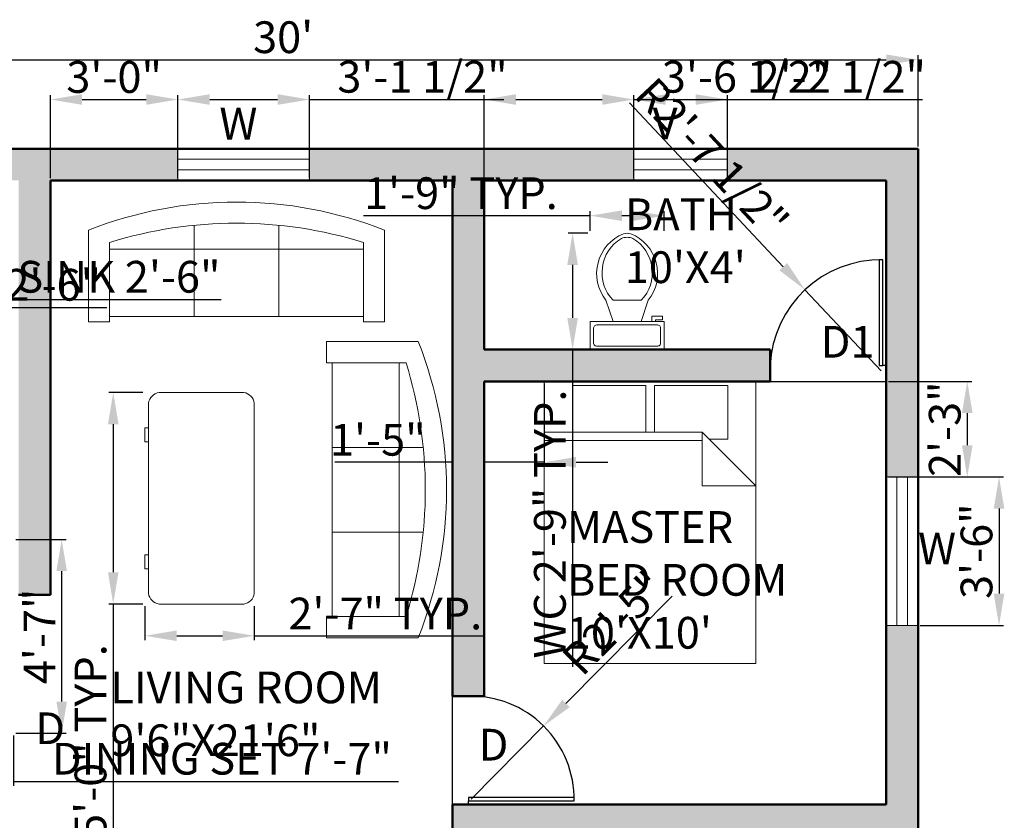
# Model space of a CAD drawing. Units: inches. Extents: x 16989 to 17950, y 7982 to 8536.
# Tile 3 of 5: x 17136 to 17415, y 8270 to 8497. Entities that reach past the tile are written whole.
import ezdxf

# ---------------------------------------------------------------- set-up
doc = ezdxf.new("R2010")
doc.units = ezdxf.units.IN
for name, color, linetype, lineweight in [('A-ANNO-DIMS', 2, 'Continuous', 18), ('A-ANNO-IDEN', 7, 'Continuous', 18), ('A-AREA-IDEN', 7, 'Continuous', 25), ('A-DOOR', 3, 'Continuous', 25), ('A-FLOR-FIXT', 9, 'Continuous', 18), ('A-FURN', 8, 'Continuous', 18), ('A-GLAZ', 4, 'Continuous', 18), ('A-WALL', 7, 'Continuous', 50)]:
    doc.layers.add(name, color=color, linetype=linetype, lineweight=lineweight)
doc.layers.add('A-WALL-PATT', color=177, linetype='Continuous', lineweight=13, true_color=0x293189)
doc.styles.get("Standard").update_dxf_attribs({"font": 'arial.ttf'})
doc.dimstyles.new('ISO-25', dxfattribs={"dimtxt": 9, "dimasz": 9, "dimexe": 1.25, "dimexo": 0.625, "dimtad": 1, "dimdec": 1, "dimrnd": 9, "dimlunit": 3, "dimtxsty": 'Standard', "dimcen": 2.5, "dimadec": 0, "dimazin": 0, "dimtfac": 1, "dimtdec": 1, "dimtmove": 0, "dimatfit": 3, "dimfxl": 1, "dimarcsym": 0})

# ---------------------------------------------------------------- blocks, each defined once
blk = doc.blocks.new('Sofa - Roundback 7 ft.')
for p, q in [((-12.00002, -32.4421), (-12.00003, -6.5971)), ((11.99997, -32.4421), (11.99998, -6.5971)), ((-36.000027, -34), (-36.000027, -11.4696)), ((-35.999844, -13.3819), (35.9998, -13.3819)), ((35.99998, -34), (35.99998, -11.4696)), ((-36.000027, -32.4421), (35.99998, -32.4421))]:
    blk.add_line(p, q)
for points in [[(-36.000027, -34), (-42.000027, -34), (-42.000027, -8)], [(41.99998, -8), (41.99998, -34), (35.99998, -34)]]:
    blk.add_lwpolyline(points)
for centre, radius, start, end in [((0, -114.25), 114.25, 68.43141, 111.5686), ((-0.00001, -127.1968), 121.1968, 72.72033, 107.2797)]:
    blk.add_arc(centre, radius, start, end)
blk = doc.blocks.new('Desk - 30 x 60 in.')
for p, q in [((-26.999995, 0), (26.999995, 0)), ((-29.999995, -27), (-29.999995, -3)), ((29.999995, -3), (29.999995, -27)), ((26.999995, -30), (-26.999995, -30)), ((-20.000005, -30), (-20.000005, -31)), ((-16.000005, -31), (-16.000005, -30)), ((15.999995, -31), (15.999995, -30)), ((19.999995, -30), (19.999995, -31)), ((-20.000005, -31), (-16.000005, -31)), ((19.999995, -31), (15.999995, -31))]:
    blk.add_line(p, q)
for centre, start, end in [((-26.499995, -3.5), 98.1301, 171.8699), ((26.499995, -3.5), 8.130102, 81.8699), ((-26.499995, -26.5), 188.1301, 261.8699), ((26.499995, -26.5), 278.1301, 351.8699)]:
    blk.add_arc(centre, 3.535534, start, end)
blk = doc.blocks.new('Bed - Queen')
for p, q in [((0, -80.00003), (0, 0)), ((0, 0), (59.99999, 0)), ((59.99999, 0), (59.99999, -80.00003)), ((7.99999, -1.2), (28.79998, -1.2)), ((7.99999, -14.4), (7.99999, -1.2)), ((28.79998, -1.2), (28.79998, -14.4)), ((31.19999, -1.2), (51.99999, -1.2)), ((31.19999, -14.4), (31.19999, -1.2)), ((51.99999, -1.2), (51.99999, -16.4)), ((0, -14.4), (44.8, -14.4)), ((59.99999, -29.6), (44.8, -14.4)), ((44.8, -14.4), (44.8, -29.6)), ((51.99999, -16.4), (46.79936, -16.4)), ((44.8, -16.8), (0, -16.8)), ((44.8, -29.6), (59.99999, -29.6)), ((59.99999, -80.00003), (0, -80.00003))]:
    blk.add_line(p, q)
blk = doc.blocks.new('Toilet - top')
for p, q in [((9.5, -6), (9.5, -2)), ((-8, -8.5), (-8, -8)), ((-7, -8), (-7, -9.5)), ((-4, -8), (-6, -14)), ((4, -8), (6, -14)), ((-10, -8.5), (-8, -8.5)), ((-10, -9.5), (-10, -8.5)), ((-7, -9.5), (-10, -9.5)), ((4, -14), (-4, -14))]:
    blk.add_line(p, q)
blk.add_lwpolyline([(10.5, -8), (10.5, 0), (-10.5, 0), (-10.5, -8)], close=True)
for points in [[(-9.5, -2), (-9.5, -6)], [(8.5, -1), (-8.5, -1)], [(-8.5, -7), (8.5, -7)]]:
    blk.add_lwpolyline(points)
for centre, radius, start, end in [((-8.62, -1.88), 0.884, 81.8699, 188.1301), ((8.62, -1.88), 0.884, 351.8699, 98.1301), ((-8.62, -6.12), 0.884, 171.8699, 278.1301), ((8.62, -6.12), 0.884, 261.8699, 8.1301), ((3.52, -21.58), 12.17, 141.4691, 247.9714), ((4.2, -21.82), 11.33, 136.3677, 238.9468), ((-3.52, -21.58), 12.17, 292.0284, 38.5307), ((-4.2, -21.82), 11.33, 301.053, 43.6321), ((0, -27.88), 4, 245.7318, 294.2682), ((0, -29), 4, 254.8605, 285.1395)]:
    blk.add_arc(centre, radius, start, end)
blk = doc.blocks.new('*D8')
at = {"layer": 'A-ANNO-DIMS', "color": 0, "lineweight": -2, "transparency": 16777216}
for p, q in [((17030.22, 8460.89), (17030.22, 8486.75)), ((17390.22, 8460.89), (17390.22, 8486.75)), ((17039.22, 8485.5), (17381.22, 8485.5))]:
    blk.add_line(p, q, dxfattribs=at)
at = {"layer": 'A-ANNO-DIMS', "color": 0, "transparency": 16777216}
for points in [[(17039.22, 8487), (17039.22, 8484), (17030.22, 8485.5)], [(17381.22, 8487), (17381.22, 8484), (17390.22, 8485.5)]]:
    blk.add_solid(points, dxfattribs=at)
at = {"layer": 'Defpoints', "color": 0, "transparency": 16777216}
for p in [(17390.22, 8485.5), (17030.22, 8460.26), (17390.22, 8460.26)]:
    blk.add_point(p, dxfattribs=at)
at = {"layer": 'A-ANNO-DIMS', "color": 0, "transparency": 16777216, "insert": (17210.22, 8490.72), "char_height": 9, "attachment_point": 5}
blk.add_mtext("30'", dxfattribs=at)
blk = doc.blocks.new('DOOR-LEAF-30IN')
for p, q in [((1, 0), (1, 30)), ((1, 30), (2, 30)), ((2, 30), (2, 0)), ((0, 0), (1, 0)), ((2, 0), (1, 0))]:
    blk.add_line(p, q)
blk = doc.blocks.new('*D23')
at = {"layer": 'A-ANNO-DIMS', "color": 0, "lineweight": -2, "transparency": 16777216}
for p, q in [((17296.61, 8436.31), (17291.03, 8436.31)), ((17292.28, 8427.31), (17292.28, 8412.26)), ((17296.61, 8403.26), (17291.03, 8403.26)), ((17292.28, 8403.26), (17292.28, 8313.34))]:
    blk.add_line(p, q, dxfattribs=at)
at = {"layer": 'A-ANNO-DIMS', "color": 0, "transparency": 16777216}
for points in [[(17290.78, 8427.31), (17293.78, 8427.31), (17292.28, 8436.31)], [(17290.78, 8412.26), (17293.78, 8412.26), (17292.28, 8403.26)]]:
    blk.add_solid(points, dxfattribs=at)
at = {"layer": 'Defpoints', "color": 0, "transparency": 16777216}
for p in [(17297.24, 8436.31), (17292.28, 8403.26), (17297.24, 8403.26)]:
    blk.add_point(p, dxfattribs=at)
at = {"layer": 'A-ANNO-DIMS', "color": 0, "transparency": 16777216, "insert": (17287, 8353.8), "char_height": 9, "attachment_point": 5, "rotation": 90}
blk.add_mtext('WC 2\'-9" TYP.', dxfattribs=at)
blk = doc.blocks.new('*D24')
at = {"layer": 'A-ANNO-DIMS', "color": 0, "lineweight": -2, "transparency": 16777216}
for p, q in [((17297.24, 8436.93), (17297.24, 8442.51)), ((17318.24, 8436.93), (17318.24, 8442.51)), ((17297.24, 8441.26), (17232.98, 8441.26)), ((17309.24, 8441.26), (17306.24, 8441.26))]:
    blk.add_line(p, q, dxfattribs=at)
at = {"layer": 'A-ANNO-DIMS', "color": 0, "transparency": 16777216}
for points in [[(17306.24, 8442.76), (17306.24, 8439.76), (17297.24, 8441.26)], [(17309.24, 8442.76), (17309.24, 8439.76), (17318.24, 8441.26)]]:
    blk.add_solid(points, dxfattribs=at)
at = {"layer": 'Defpoints', "color": 0, "transparency": 16777216}
for p in [(17297.24, 8441.26), (17297.24, 8436.31), (17318.24, 8436.31)]:
    blk.add_point(p, dxfattribs=at)
at = {"layer": 'A-ANNO-DIMS', "color": 0, "transparency": 16777216, "insert": (17260.61, 8446.48), "char_height": 9, "attachment_point": 5}
blk.add_mtext('1\'-9" TYP.', dxfattribs=at)
blk = doc.blocks.new('*D27')
at = {"layer": 'A-ANNO-DIMS', "color": 0, "lineweight": -2, "transparency": 16777216}
for p, q in [((17170.41, 8391.11), (17160.79, 8391.11)), ((17162.04, 8382.11), (17162.04, 8340.11)), ((17170.41, 8331.11), (17160.79, 8331.11)), ((17162.04, 8331.11), (17162.04, 8228.71))]:
    blk.add_line(p, q, dxfattribs=at)
at = {"layer": 'A-ANNO-DIMS', "color": 0, "transparency": 16777216}
for points in [[(17160.54, 8382.11), (17163.54, 8382.11), (17162.04, 8391.11)], [(17160.54, 8340.11), (17163.54, 8340.11), (17162.04, 8331.11)]]:
    blk.add_solid(points, dxfattribs=at)
at = {"layer": 'Defpoints', "color": 0, "transparency": 16777216}
for p in [(17171.04, 8391.11), (17162.04, 8331.11), (17171.04, 8331.11)]:
    blk.add_point(p, dxfattribs=at)
at = {"layer": 'A-ANNO-DIMS', "color": 0, "transparency": 16777216, "insert": (17156.76, 8275.41), "char_height": 9, "attachment_point": 5, "rotation": 90}
blk.add_mtext('DESK 5\'-0" TYP.', dxfattribs=at)
blk = doc.blocks.new('*D28')
at = {"layer": 'A-ANNO-DIMS', "color": 0, "lineweight": -2, "transparency": 16777216}
for p, q in [((17171.04, 8330.48), (17171.04, 8320.86)), ((17202.04, 8330.48), (17202.04, 8320.86)), ((17180.04, 8322.11), (17193.04, 8322.11)), ((17202.04, 8322.11), (17267.3, 8322.11))]:
    blk.add_line(p, q, dxfattribs=at)
at = {"layer": 'A-ANNO-DIMS', "color": 0, "transparency": 16777216}
for points in [[(17180.04, 8323.61), (17180.04, 8320.61), (17171.04, 8322.11)], [(17193.04, 8323.61), (17193.04, 8320.61), (17202.04, 8322.11)]]:
    blk.add_solid(points, dxfattribs=at)
at = {"layer": 'Defpoints', "color": 0, "transparency": 16777216}
for p in [(17171.04, 8331.11), (17202.04, 8331.11), (17202.04, 8322.11)]:
    blk.add_point(p, dxfattribs=at)
at = {"layer": 'A-ANNO-DIMS', "color": 0, "transparency": 16777216, "insert": (17239.17, 8327.25), "char_height": 9, "attachment_point": 5}
blk.add_mtext('2\'-7" TYP.', dxfattribs=at)
blk = doc.blocks.new('*D29')
at = {"layer": 'A-ANNO-DIMS', "color": 0, "lineweight": -2, "transparency": 16777216}
for p, q in [((17048.3, 8419.09), (17048.3, 8413.96)), ((17078.3, 8419.09), (17078.3, 8413.96)), ((17057.3, 8415.21), (17069.3, 8415.21)), ((17078.3, 8415.21), (17160.21, 8415.21))]:
    blk.add_line(p, q, dxfattribs=at)
at = {"layer": 'A-ANNO-DIMS', "color": 0, "transparency": 16777216}
for points in [[(17057.3, 8416.71), (17057.3, 8413.71), (17048.3, 8415.21)], [(17069.3, 8416.71), (17069.3, 8413.71), (17078.3, 8415.21)]]:
    blk.add_solid(points, dxfattribs=at)
at = {"layer": 'Defpoints', "color": 0, "transparency": 16777216}
for p in [(17048.3, 8419.71), (17078.3, 8419.71), (17078.3, 8415.21)]:
    blk.add_point(p, dxfattribs=at)
at = {"layer": 'A-ANNO-DIMS', "color": 0, "transparency": 16777216, "insert": (17123.75, 8420.49), "char_height": 9, "attachment_point": 5}
blk.add_mtext('RANGE 2\'-6"', dxfattribs=at)
blk = doc.blocks.new('*D31')
at = {"layer": 'A-ANNO-DIMS', "color": 0, "lineweight": -2, "transparency": 16777216}
for p, q in [((17095.68, 8421.36), (17095.68, 8416.24)), ((17125.68, 8421.36), (17125.68, 8416.24)), ((17104.68, 8417.49), (17116.68, 8417.49)), ((17125.68, 8417.49), (17192.65, 8417.49))]:
    blk.add_line(p, q, dxfattribs=at)
at = {"layer": 'A-ANNO-DIMS', "color": 0, "transparency": 16777216}
for points in [[(17104.68, 8418.99), (17104.68, 8415.99), (17095.68, 8417.49)], [(17116.68, 8418.99), (17116.68, 8415.99), (17125.68, 8417.49)]]:
    blk.add_solid(points, dxfattribs=at)
at = {"layer": 'Defpoints', "color": 0, "transparency": 16777216}
for p in [(17095.68, 8421.99), (17125.68, 8421.99), (17125.68, 8417.49)]:
    blk.add_point(p, dxfattribs=at)
at = {"layer": 'A-ANNO-DIMS', "color": 0, "transparency": 16777216, "insert": (17163.66, 8422.77), "char_height": 9, "attachment_point": 5}
blk.add_mtext('SINK 2\'-6"', dxfattribs=at)
blk = doc.blocks.new('*D33')
at = {"layer": 'A-ANNO-DIMS', "color": 0, "lineweight": -2, "transparency": 16777216}
for p, q in [((17042.78, 8293.82), (17042.78, 8279.54)), ((17133.78, 8293.82), (17133.78, 8279.54)), ((17051.78, 8280.79), (17124.78, 8280.79)), ((17133.78, 8280.79), (17242.95, 8280.79))]:
    blk.add_line(p, q, dxfattribs=at)
at = {"layer": 'A-ANNO-DIMS', "color": 0, "transparency": 16777216}
for points in [[(17051.78, 8282.29), (17051.78, 8279.29), (17042.78, 8280.79)], [(17124.78, 8282.29), (17124.78, 8279.29), (17133.78, 8280.79)]]:
    blk.add_solid(points, dxfattribs=at)
at = {"layer": 'Defpoints', "color": 0, "transparency": 16777216}
for p in [(17042.78, 8294.44), (17133.78, 8294.44), (17133.78, 8280.79)]:
    blk.add_point(p, dxfattribs=at)
at = {"layer": 'A-ANNO-DIMS', "color": 0, "transparency": 16777216, "insert": (17192.87, 8286.07), "char_height": 9, "attachment_point": 5}
blk.add_mtext('DINING SET 7\'-7"', dxfattribs=at)
blk = doc.blocks.new('*D34')
at = {"layer": 'A-ANNO-DIMS', "color": 0, "lineweight": -2, "transparency": 16777216}
for p, q in [((17134.41, 8349.44), (17148.68, 8349.44)), ((17147.43, 8303.44), (17147.43, 8340.44)), ((17134.41, 8294.44), (17148.68, 8294.44))]:
    blk.add_line(p, q, dxfattribs=at)
at = {"layer": 'A-ANNO-DIMS', "color": 0, "transparency": 16777216}
for points in [[(17145.93, 8340.44), (17148.93, 8340.44), (17147.43, 8349.44)], [(17145.93, 8303.44), (17148.93, 8303.44), (17147.43, 8294.44)]]:
    blk.add_solid(points, dxfattribs=at)
at = {"layer": 'Defpoints', "color": 0, "transparency": 16777216}
for p in [(17133.78, 8349.44), (17147.43, 8349.44), (17133.78, 8294.44)]:
    blk.add_point(p, dxfattribs=at)
at = {"layer": 'A-ANNO-DIMS', "color": 0, "transparency": 16777216, "insert": (17142.31, 8321.94), "char_height": 9, "attachment_point": 5, "rotation": 90}
blk.add_mtext('4\'-7"', dxfattribs=at)
blk = doc.blocks.new('*D37')
at = {"layer": 'A-ANNO-DIMS', "color": 0, "lineweight": -2, "transparency": 16777216}
for p, q in [((17144.22, 8451.89), (17144.22, 8475.46)), ((17180.39, 8451.89), (17180.39, 8475.46)), ((17153.22, 8474.21), (17171.39, 8474.21))]:
    blk.add_line(p, q, dxfattribs=at)
at = {"layer": 'A-ANNO-DIMS', "color": 0, "transparency": 16777216}
for points in [[(17153.22, 8475.71), (17153.22, 8472.71), (17144.22, 8474.21)], [(17171.39, 8475.71), (17171.39, 8472.71), (17180.39, 8474.21)]]:
    blk.add_solid(points, dxfattribs=at)
at = {"layer": 'Defpoints', "color": 0, "transparency": 16777216}
for p in [(17180.39, 8474.21), (17144.22, 8451.26), (17180.39, 8451.26)]:
    blk.add_point(p, dxfattribs=at)
at = {"layer": 'A-ANNO-DIMS', "color": 0, "transparency": 16777216, "insert": (17162.31, 8479.43), "char_height": 9, "attachment_point": 5}
blk.add_mtext('3\'-0"', dxfattribs=at)
blk = doc.blocks.new('*D38')
at = {"layer": 'A-ANNO-DIMS', "color": 0, "lineweight": -2, "transparency": 16777216}
for p, q in [((17180.39, 8451.89), (17180.39, 8475.46)), ((17217.66, 8451.89), (17217.66, 8475.46)), ((17189.39, 8474.21), (17208.66, 8474.21)), ((17217.66, 8474.21), (17272.8, 8474.21))]:
    blk.add_line(p, q, dxfattribs=at)
at = {"layer": 'A-ANNO-DIMS', "color": 0, "transparency": 16777216}
for points in [[(17189.39, 8475.71), (17189.39, 8472.71), (17180.39, 8474.21)], [(17208.66, 8475.71), (17208.66, 8472.71), (17217.66, 8474.21)]]:
    blk.add_solid(points, dxfattribs=at)
at = {"layer": 'Defpoints', "color": 0, "transparency": 16777216}
for p in [(17217.66, 8474.21), (17180.39, 8451.26), (17217.66, 8451.26)]:
    blk.add_point(p, dxfattribs=at)
at = {"layer": 'A-ANNO-DIMS', "color": 0, "transparency": 16777216, "insert": (17249.73, 8479.49), "char_height": 9, "attachment_point": 5}
blk.add_mtext('3\'-1 1/2"', dxfattribs=at)
blk = doc.blocks.new('*D39')
at = {"layer": 'A-ANNO-DIMS', "color": 0, "lineweight": -2, "transparency": 16777216}
for p, q in [((17267.22, 8451.89), (17267.22, 8475.46)), ((17309.67, 8451.89), (17309.67, 8475.46)), ((17276.22, 8474.21), (17300.67, 8474.21)), ((17309.67, 8474.21), (17364.81, 8474.21))]:
    blk.add_line(p, q, dxfattribs=at)
at = {"layer": 'A-ANNO-DIMS', "color": 0, "transparency": 16777216}
for points in [[(17276.22, 8475.71), (17276.22, 8472.71), (17267.22, 8474.21)], [(17300.67, 8475.71), (17300.67, 8472.71), (17309.67, 8474.21)]]:
    blk.add_solid(points, dxfattribs=at)
at = {"layer": 'Defpoints', "color": 0, "transparency": 16777216}
for p in [(17309.67, 8474.21), (17267.22, 8451.26), (17309.67, 8451.26)]:
    blk.add_point(p, dxfattribs=at)
at = {"layer": 'A-ANNO-DIMS', "color": 0, "transparency": 16777216, "insert": (17341.74, 8479.49), "char_height": 9, "attachment_point": 5}
blk.add_mtext('3\'-6 1/2"', dxfattribs=at)
blk = doc.blocks.new('*D40')
at = {"layer": 'A-ANNO-DIMS', "color": 0, "lineweight": -2, "transparency": 16777216}
for p, q in [((17309.67, 8451.89), (17309.67, 8475.46)), ((17336.17, 8451.89), (17336.17, 8475.46)), ((17318.67, 8474.21), (17327.17, 8474.21)), ((17336.17, 8474.21), (17391.47, 8474.21))]:
    blk.add_line(p, q, dxfattribs=at)
at = {"layer": 'A-ANNO-DIMS', "color": 0, "transparency": 16777216}
for points in [[(17318.67, 8475.71), (17318.67, 8472.71), (17309.67, 8474.21)], [(17327.17, 8475.71), (17327.17, 8472.71), (17336.17, 8474.21)]]:
    blk.add_solid(points, dxfattribs=at)
at = {"layer": 'Defpoints', "color": 0, "transparency": 16777216}
for p in [(17336.17, 8474.21), (17309.67, 8451.26), (17336.17, 8451.26)]:
    blk.add_point(p, dxfattribs=at)
at = {"layer": 'A-ANNO-DIMS', "color": 0, "transparency": 16777216, "insert": (17368.32, 8479.49), "char_height": 9, "attachment_point": 5}
blk.add_mtext('2\'-2 1/2"', dxfattribs=at)
blk = doc.blocks.new('*D41')
at = {"layer": 'A-ANNO-DIMS', "color": 0, "lineweight": -2, "transparency": 16777216}
for p, q in [((17381.84, 8394.26), (17405.42, 8394.26)), ((17404.17, 8385.26), (17404.17, 8376.17)), ((17381.84, 8367.17), (17405.42, 8367.17))]:
    blk.add_line(p, q, dxfattribs=at)
at = {"layer": 'A-ANNO-DIMS', "color": 0, "transparency": 16777216}
for points in [[(17402.67, 8385.26), (17405.67, 8385.26), (17404.17, 8394.26)], [(17402.67, 8376.17), (17405.67, 8376.17), (17404.17, 8367.17)]]:
    blk.add_solid(points, dxfattribs=at)
at = {"layer": 'Defpoints', "color": 0, "transparency": 16777216}
for p in [(17381.22, 8394.26), (17381.22, 8367.17), (17404.17, 8367.17)]:
    blk.add_point(p, dxfattribs=at)
at = {"layer": 'A-ANNO-DIMS', "color": 0, "transparency": 16777216, "insert": (17398.95, 8380.71), "char_height": 9, "attachment_point": 5, "rotation": 90}
blk.add_mtext('2\'-3"', dxfattribs=at)
blk = doc.blocks.new('*D42')
at = {"layer": 'A-ANNO-DIMS', "color": 0, "lineweight": -2, "transparency": 16777216}
for p, q in [((17390.84, 8367.17), (17414.42, 8367.17)), ((17413.17, 8358.17), (17413.17, 8334.05)), ((17390.84, 8325.05), (17414.42, 8325.05))]:
    blk.add_line(p, q, dxfattribs=at)
at = {"layer": 'A-ANNO-DIMS', "color": 0, "transparency": 16777216}
for points in [[(17411.67, 8358.17), (17414.67, 8358.17), (17413.17, 8367.17)], [(17411.67, 8334.05), (17414.67, 8334.05), (17413.17, 8325.05)]]:
    blk.add_solid(points, dxfattribs=at)
at = {"layer": 'Defpoints', "color": 0, "transparency": 16777216}
for p in [(17390.22, 8367.17), (17390.22, 8325.05), (17413.17, 8325.05)]:
    blk.add_point(p, dxfattribs=at)
at = {"layer": 'A-ANNO-DIMS', "color": 0, "transparency": 16777216, "insert": (17407.95, 8346.11), "char_height": 9, "attachment_point": 5, "rotation": 90}
blk.add_mtext('3\'-6"', dxfattribs=at)
blk = doc.blocks.new('*D68')
at = {"layer": 'A-ANNO-DIMS', "color": 0, "lineweight": -2, "transparency": 16777216}
for p, q in [((17267.22, 8393.64), (17267.22, 8370.06)), ((17284.25, 8393.64), (17284.25, 8370.06)), ((17258.22, 8371.31), (17224.89, 8371.31)), ((17284.25, 8371.31), (17267.22, 8371.31)), ((17293.25, 8371.31), (17302.25, 8371.31))]:
    blk.add_line(p, q, dxfattribs=at)
at = {"layer": 'A-ANNO-DIMS', "color": 0, "transparency": 16777216}
for points in [[(17258.22, 8372.81), (17258.22, 8369.81), (17267.22, 8371.31)], [(17293.25, 8372.81), (17293.25, 8369.81), (17284.25, 8371.31)]]:
    blk.add_solid(points, dxfattribs=at)
at = {"layer": 'Defpoints', "color": 0, "transparency": 16777216}
for p in [(17267.22, 8394.26), (17284.25, 8394.26), (17267.22, 8371.31)]:
    blk.add_point(p, dxfattribs=at)
at = {"layer": 'A-ANNO-DIMS', "color": 0, "transparency": 16777216, "insert": (17237.06, 8376.53), "char_height": 9, "attachment_point": 5}
blk.add_mtext('1\'-5"', dxfattribs=at)
blk = doc.blocks.new('*D73')
at = {"layer": 'A-ANNO-DIMS', "color": 0, "lineweight": -2, "transparency": 16777216}
for p, q in [((17308.37, 8473.28), (17352, 8426.79)), ((17379.72, 8397.27), (17358.16, 8420.23))]:
    blk.add_line(p, q, dxfattribs=at)
at = {"layer": 'A-ANNO-DIMS', "color": 0, "transparency": 16777216}
blk.add_solid([(17353.1, 8427.82), (17350.91, 8425.77), (17358.16, 8420.23)], dxfattribs=at)
at = {"layer": 'Defpoints', "color": 0, "transparency": 16777216}
for p in [(17358.16, 8420.23), (17379.72, 8397.27)]:
    blk.add_point(p, dxfattribs=at)
at = {"layer": 'A-ANNO-DIMS', "color": 0, "transparency": 16777216, "insert": (17330.96, 8456.93), "char_height": 9, "attachment_point": 5, "rotation": 313.1866}
blk.add_mtext('R2\'-7 1/2"', dxfattribs=at)
blk = doc.blocks.new('*D75')
at = {"layer": 'A-ANNO-DIMS', "color": 0, "lineweight": -2, "transparency": 16777216}
for p, q in [((17320.51, 8333.32), (17290.4, 8302.92)), ((17263.49, 8275.76), (17284.07, 8296.53))]:
    blk.add_line(p, q, dxfattribs=at)
at = {"layer": 'A-ANNO-DIMS', "color": 0, "transparency": 16777216}
blk.add_solid([(17289.33, 8303.98), (17291.46, 8301.86), (17284.07, 8296.53)], dxfattribs=at)
at = {"layer": 'Defpoints', "color": 0, "transparency": 16777216}
for p in [(17284.07, 8296.53), (17263.49, 8275.76)]:
    blk.add_point(p, dxfattribs=at)
at = {"layer": 'A-ANNO-DIMS', "color": 0, "transparency": 16777216, "insert": (17304.91, 8324.99), "char_height": 9, "attachment_point": 5, "rotation": 45.2673}
blk.add_mtext('R2\'-5"', dxfattribs=at)

msp = doc.modelspace()

# ---------------------------------------------------------------- hatches: boundary and pattern name
at = {"layer": 'A-WALL-PATT'}
h = msp.add_hatch(color=256, dxfattribs=at)
h.dxf.hatch_style = 1
h.paths.add_polyline_path([(17039.22, 8310.16), (17030.22, 8310.16), (17030.22, 8100.26), (17049.62, 8100.26), (17049.62, 8109.26), (17039.22, 8109.26), (17039.22, 8256.26), (17144.22, 8256.26), (17144.22, 8265.26), (17039.22, 8265.26)])
h.paths.add_polyline_path([(17039.22, 8451.26), (17065.89, 8451.26), (17065.89, 8460.26), (17030.22, 8460.26), (17030.22, 8357.88), (17039.22, 8357.88)])
h.paths.add_polyline_path([(17180.39, 8460.26), (17105.01, 8460.26), (17105.01, 8451.26), (17135.22, 8451.26), (17135.22, 8333.76), (17144.22, 8333.76), (17144.22, 8451.26), (17180.39, 8451.26)])
h.paths.add_polyline_path([(17309.67, 8460.26), (17217.66, 8460.26), (17217.66, 8451.26), (17258.22, 8451.26), (17258.22, 8304.98), (17262.72, 8304.98, -0.013209), (17264.26, 8304.98), (17267.22, 8304.98), (17267.22, 8394.26), (17348.26, 8394.26), (17348.26, 8403.26), (17267.22, 8403.26), (17267.22, 8451.26), (17309.67, 8451.26)])
h.paths.add_polyline_path([(17390.22, 8460.26), (17336.17, 8460.26), (17336.17, 8451.26), (17381.22, 8451.26), (17381.22, 8403.26), (17381.22, 8394.26), (17381.22, 8367.17), (17390.22, 8367.17)])
h.paths.add_polyline_path([(17390.22, 8325.05), (17381.22, 8325.05), (17381.22, 8274.26), (17267.22, 8274.26), (17258.22, 8274.26), (17258.22, 8265.26), (17267.22, 8265.26), (17381.22, 8265.26), (17381.22, 8238), (17390.22, 8238)])
h.paths.add_polyline_path([(17390.22, 8194.87), (17381.22, 8194.87), (17381.22, 8157.26), (17381.22, 8148.26), (17381.22, 8109.26), (17332.58, 8109.26), (17332.58, 8100.26), (17390.22, 8100.26)])
h.paths.add_polyline_path([(17349.64, 8157.26), (17267.22, 8157.26), (17267.22, 8231.5), (17258.22, 8231.5), (17258.22, 8193.26), (17144.22, 8193.26), (17114.21, 8193.26), (17114.21, 8184.26), (17144.22, 8184.26), (17258.22, 8184.26), (17258.22, 8109.26), (17088.6, 8109.26), (17088.6, 8100.26), (17308.63, 8100.26), (17308.63, 8109.26), (17267.22, 8109.26), (17267.22, 8148.26), (17349.64, 8148.26)])

# ---------------------------------------------------------------- linework, layer by layer
at = {"layer": 'A-DOOR'}
for p, q in [((17348.26, 8394.26), (17381.22, 8394.26)), ((17258.22, 8274.26), (17258.22, 8304.98))]:
    msp.add_line(p, q, dxfattribs=at)
for centre, radius, start, end in [((17379.72, 8397.27), 31.5, 89.0904, 177.282), ((17263.49, 8275.76), 29.23, 359.0199, 91.5135)]:
    msp.add_arc(centre, radius, start, end, dxfattribs=at)
at = {"layer": 'A-GLAZ'}
for p, q in [((17180.39, 8460.26), (17180.39, 8451.26)), ((17217.66, 8460.26), (17217.66, 8451.26)), ((17309.67, 8460.26), (17309.67, 8451.26)), ((17336.17, 8460.26), (17336.17, 8451.26)), ((17217.66, 8457.26), (17180.39, 8457.26)), ((17336.17, 8457.26), (17309.67, 8457.26)), ((17217.66, 8454.26), (17180.39, 8454.26)), ((17336.17, 8454.26), (17309.67, 8454.26)), ((17390.22, 8367.17), (17381.22, 8367.17)), ((17384.22, 8325.05), (17384.22, 8367.17)), ((17387.22, 8325.05), (17387.22, 8367.17)), ((17390.22, 8325.05), (17381.22, 8325.05))]:
    msp.add_line(p, q, dxfattribs=at)
at = {"layer": 'A-WALL'}
for p, q in [((17390.22, 8460.26), (17030.22, 8460.26)), ((17390.22, 8100.26), (17390.22, 8460.26)), ((17144.22, 8451.26), (17144.22, 8333.76)), ((17258.22, 8451.26), (17144.22, 8451.26)), ((17258.22, 8451.26), (17258.22, 8304.98)), ((17381.22, 8451.26), (17267.22, 8451.26)), ((17267.22, 8451.26), (17267.22, 8403.26)), ((17381.22, 8403.26), (17381.22, 8451.26)), ((17348.26, 8403.26), (17267.22, 8403.26)), ((17348.26, 8403.26), (17348.26, 8394.26)), ((17381.22, 8403.26), (17381.22, 8394.26)), ((17348.26, 8394.26), (17267.22, 8394.26)), ((17267.22, 8394.26), (17267.22, 8304.98)), ((17381.22, 8274.26), (17381.22, 8394.26)), ((17381.22, 8274.26), (17381.22, 8394.26)), ((17144.22, 8333.76), (17135.22, 8333.76)), ((17267.22, 8304.98), (17258.22, 8304.98)), ((17267.22, 8274.26), (17258.22, 8274.26)), ((17258.22, 8274.26), (17258.22, 8265.26)), ((17381.22, 8274.26), (17267.22, 8274.26))]:
    msp.add_line(p, q, dxfattribs=at)

# ---------------------------------------------------------------- block references
at = {"layer": 'A-DOOR', "extrusion": (0, 0, -1), "zscale": -1}
msp.add_blockref('DOOR-LEAF-30IN', (-17381.22, 8398.76), dxfattribs=at)
at = {"layer": 'A-DOOR', "extrusion": (0, 0, -1), "zscale": -1, "rotation": 90.00000000000566}
msp.add_blockref('DOOR-LEAF-30IN', (-17262.72, 8274.26), dxfattribs=at)
at = {"layer": 'A-FLOR-FIXT', "rotation": 180}
msp.add_blockref('Toilet - top', (17307.74, 8403.26), dxfattribs=at)
at = {"layer": 'A-FURN'}
for name, p in [('Sofa - Roundback 7 ft.', (17196.99, 8445.14)), ('Bed - Queen', (17284.25, 8394.26))]:
    msp.add_blockref(name, p, dxfattribs=at)
at = {"layer": 'A-FURN', "rotation": 270}
for name, p in [('Sofa - Roundback 7 ft.', (17256.52, 8363.54)), ('Desk - 30 x 60 in.', (17202.04, 8361.11))]:
    msp.add_blockref(name, p, dxfattribs=at)

# ---------------------------------------------------------------- texts
at = {"layer": 'A-ANNO-IDEN', "char_height": 9, "attachment_point": 1}
for s, insert in [('W', (17192.13, 8471.87)), ('V', (17314.97, 8471.9)), ('D1', (17362.6, 8409.99)), ('W', (17390.22, 8351.39)), ('D', (17139.92, 8300.37)), ('D', (17265.63, 8295.71))]:
    msp.add_mtext_dynamic_manual_height_columns(s, width=19.3379, gutter_width=12.5, heights=[0], dxfattribs=dict(at, insert=insert))
at = {"layer": 'A-AREA-IDEN', "char_height": 9, "attachment_point": 1}
for s, width, insert in [("BATH\\P10'X4'", 65.8099, (17307.09, 8446.15)), ("MASTER\\PBED ROOM\\P10'X10'", 77.3711, (17290.65, 8357.46)), ('LIVING ROOM\\P9\'6"X21\'6"', 95.549, (17161.21, 8311.96))]:
    msp.add_mtext_dynamic_manual_height_columns(s, width=width, gutter_width=12.5, heights=[0], dxfattribs=dict(at, insert=insert))

# ---------------------------------------------------------------- dimensions: what is measured, and where the dimension line sits
at = {"layer": 'A-ANNO-DIMS'}
for base, p1, p2, override, picture, middle in [((17390.22, 8485.5), (17030.22, 8460.26), (17390.22, 8460.26), {"dimclrd": 0, "dimclre": 0, "dimclrt": 0}, '*D8', (17210.22, 8490.72)), ((17217.66, 8474.21), (17180.39, 8451.26), (17217.66, 8451.26), {"dimdec": 1, "dimlfac": 1, "dimrnd": 0, "dimzin": 1, "dimdsep": 46, "dimlunit": 4, "dimfrac": 2}, '*D38', (17249.73, 8479.49)), ((17336.17, 8474.21), (17309.67, 8451.26), (17336.17, 8451.26), {"dimdec": 1, "dimlfac": 1, "dimrnd": 0, "dimzin": 1, "dimdsep": 46, "dimlunit": 4, "dimfrac": 2}, '*D40', (17368.32, 8479.49)), ((17180.39, 8474.21), (17144.22, 8451.26), (17180.39, 8451.26), {"dimdec": 1, "dimlfac": 1, "dimrnd": 0, "dimzin": 1, "dimdsep": 46, "dimlunit": 4, "dimfrac": 2}, '*D37', (17162.31, 8479.43))]:
    dim = msp.add_linear_dim(base=base, p1=p1, p2=p2, dimstyle='ISO-25', override=override, dxfattribs=at)
    dim.commit()
    dim.dimension.update_dxf_attribs({"geometry": picture, "text_midpoint": middle})
for base, p1, p2, angle, picture, middle in [((17309.67, 8474.2106), (17267.2194, 8451.2606), (17309.67, 8451.2606), 0, '*D39', (17341.7397, 8479.4922)), ((17267.22, 8371.31), (17284.25, 8394.26), (17267.22, 8394.26), 180, '*D68', (17237.06, 8376.53)), ((17404.17, 8367.17), (17381.22, 8394.26), (17381.22, 8367.17), 270, '*D41', (17398.95, 8380.71)), ((17413.17, 8325.05), (17390.22, 8367.17), (17390.22, 8325.05), 90, '*D42', (17407.95, 8346.11)), ((17147.43, 8349.44), (17133.78, 8294.44), (17133.78, 8349.44), 90, '*D34', (17142.31, 8321.94))]:
    dim = msp.add_linear_dim(base=base, p1=p1, p2=p2, angle=angle, dimstyle='ISO-25', override={"dimdec": 1, "dimlfac": 1, "dimrnd": 0, "dimzin": 1, "dimdsep": 46, "dimlunit": 4, "dimfrac": 2}, dxfattribs=at)
    dim.commit()
    dim.dimension.update_dxf_attribs({"geometry": picture, "text_midpoint": middle})
for center, mpoint, picture, middle in [((17379.72, 8397.27), (17358.16, 8420.23), '*D73', (17330.96, 8456.93)), ((17263.49, 8275.76), (17284.07, 8296.53), '*D75', (17304.91, 8324.99))]:
    dim = msp.add_radius_dim(center=center, mpoint=mpoint, dimstyle='ISO-25', override={"dimdec": 1, "dimlfac": 1, "dimrnd": 0, "dimzin": 1, "dimdsep": 46, "dimlunit": 4, "dimfrac": 2}, dxfattribs=at)
    dim.commit()
    dim.dimension.update_dxf_attribs({"geometry": picture, "text_midpoint": middle})
for base, p1, p2, angle, text, picture, middle in [((17297.24, 8441.26), (17318.24, 8436.31), (17297.24, 8436.31), 180, '<> TYP.', '*D24', (17260.61, 8446.48)), ((17292.2814, 8403.2606), (17297.2383, 8436.3069), (17297.2383, 8403.2606), 270, 'WC <> TYP.', '*D23', (17287.0029, 8353.8017)), ((17162.04, 8331.11), (17171.04, 8391.11), (17171.04, 8331.11), 270, 'DESK <> TYP.', '*D27', (17156.76, 8275.41))]:
    dim = msp.add_linear_dim(base=base, p1=p1, p2=p2, angle=angle, text=text, dimstyle='ISO-25', override={"dimdec": 1, "dimlfac": 1, "dimrnd": 0, "dimzin": 1, "dimdsep": 46, "dimlunit": 4, "dimfrac": 2}, dxfattribs=at)
    dim.commit()
    dim.dimension.update_dxf_attribs({"geometry": picture, "text_midpoint": middle})
for base, p1, p2, text, picture, middle in [((17125.68, 8417.49), (17095.68, 8421.99), (17125.68, 8421.99), 'SINK <>', '*D31', (17163.66, 8422.77)), ((17078.3, 8415.21), (17048.3, 8419.71), (17078.3, 8419.71), 'RANGE <>', '*D29', (17123.75, 8420.49)), ((17202.04, 8322.11), (17171.04, 8331.11), (17202.04, 8331.11), '<> TYP.', '*D28', (17239.17, 8327.25)), ((17133.78, 8280.79), (17042.78, 8294.44), (17133.78, 8294.44), 'DINING SET <>', '*D33', (17192.87, 8286.07))]:
    dim = msp.add_linear_dim(base=base, p1=p1, p2=p2, text=text, dimstyle='ISO-25', override={"dimdec": 1, "dimlfac": 1, "dimrnd": 0, "dimzin": 1, "dimdsep": 46, "dimlunit": 4, "dimfrac": 2}, dxfattribs=at)
    dim.commit()
    dim.dimension.update_dxf_attribs({"geometry": picture, "text_midpoint": middle})

doc.saveas('drawing.dxf')
